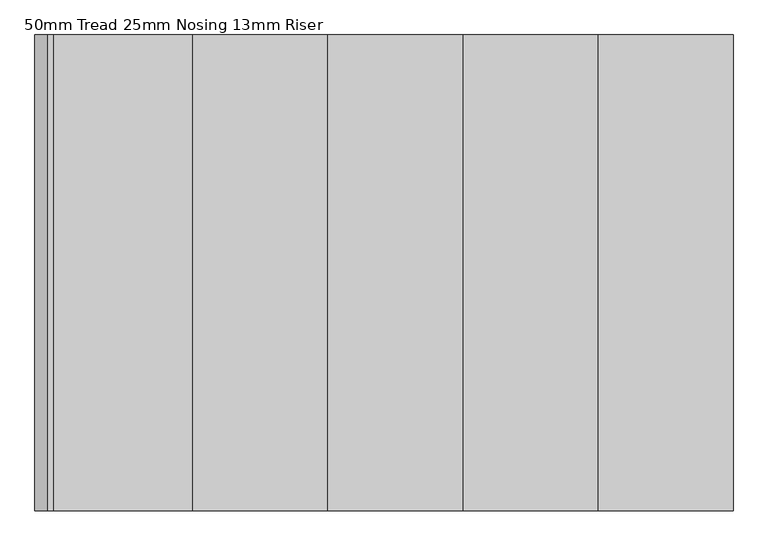
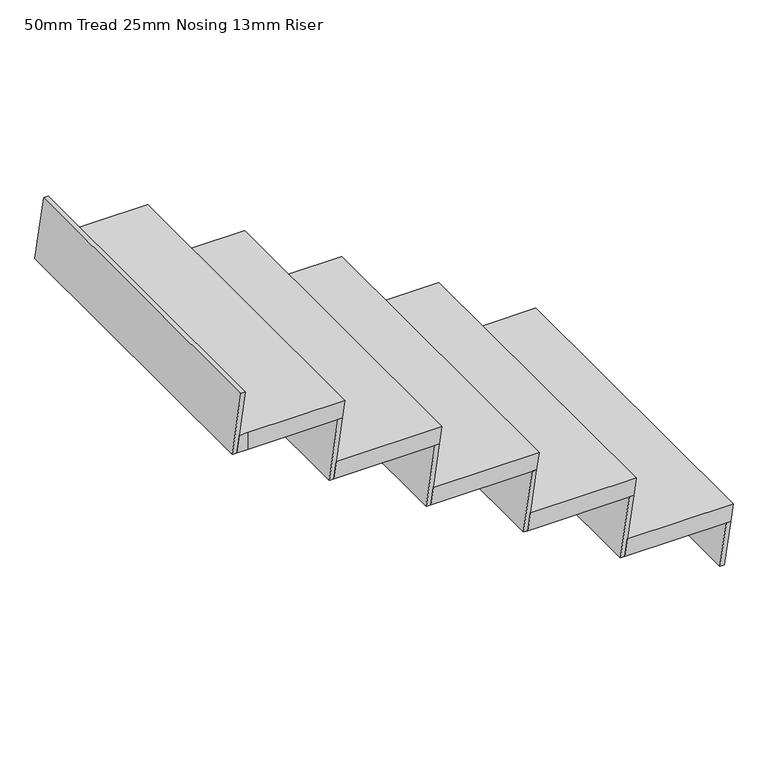
"""IFC4 building model written with IfcOpenShell, lengths in millimetres: stair flight geometry, 50mm Tread 25mm Nosing 13mm Riser."""

from ifc_helpers import new_model, si_unit, origin, place, context, project, spatial, faceted_brep, source, transform, mapped, element, save


def stair_flight_50mm_tread_25mm_nosing_13mm_riser_d346f2b6(model_context):
    return source(origin(), model_context, "Body", "Brep", [
        faceted_brep([(-839.0915237, 1810.8567276, 173.9130435), (-846.2790237, 1810.8567276, 123.9130435), (-846.2790237, 843.0180557, 123.9130435), (-839.0915237, 843.0180557, 173.9130435), (-539.0915237, 843.0180557, 173.9130435), (-539.0915237, 1810.8567276, 173.9130435), (-546.2790237, 1810.8567276, 123.9130435), (-546.2790237, 843.0180557, 123.9130435)], [[[0, 1, 2, 3]], [[3, 4, 5, 0]], [[2, 1, 6, 7]], [[4, 3, 2, 7]], [[0, 5, 6, 1]], [[5, 4, 7, 6]]]),
        faceted_brep([(-546.2790237, 1810.8567276, 123.9130435), (-564.0915237, 1810.8567276, 0.0), (-576.7200137, 1810.8567276, 0.0), (-558.9075137, 1810.8567276, 123.9130435), (-546.2790237, 843.0180557, 123.9130435), (-558.9075137, 843.0180557, 123.9130435), (-576.7200137, 843.0180557, 0.0), (-564.0915237, 843.0180557, 0.0)], [[[0, 1, 2, 3]], [[4, 5, 6, 7]], [[1, 0, 4, 7]], [[2, 1, 7, 6]], [[3, 2, 6, 5]], [[0, 3, 5, 4]]]),
        faceted_brep([(-821.2790237, 1810.8567276, 297.826087), (-846.2790237, 1810.8567276, 123.9130435), (-858.9075137, 1810.8567276, 123.9130435), (-833.9075137, 1810.8567276, 297.826087), (-821.2790237, 843.0180557, 297.826087), (-833.9075137, 843.0180557, 297.826087), (-858.9075137, 843.0180557, 123.9130435), (-846.2790237, 843.0180557, 123.9130435)], [[[0, 1, 2, 3]], [[4, 5, 6, 7]], [[1, 0, 4, 7]], [[2, 1, 7, 6]], [[3, 2, 6, 5]], [[0, 3, 5, 4]]]),
        faceted_brep([(-1114.0915237, 843.0180557, 347.826087), (-814.0915237, 843.0180557, 347.826087), (-814.0915237, 1810.8567276, 347.826087), (-1114.0915237, 1810.8567276, 347.826087), (-1121.2790237, 843.0180557, 297.826087), (-1121.2790237, 1810.8567276, 297.826087), (-821.2790237, 1810.8567276, 297.826087), (-821.2790237, 843.0180557, 297.826087)], [[[0, 1, 2, 3]], [[4, 5, 6, 7]], [[1, 0, 4, 7]], [[3, 2, 6, 5]], [[3, 5, 4, 0]], [[2, 1, 7, 6]]]),
        faceted_brep([(-1096.2790237, 1810.8567276, 471.7391304), (-1121.2790237, 1810.8567276, 297.826087), (-1133.9075137, 1810.8567276, 297.826087), (-1108.9075137, 1810.8567276, 471.7391304), (-1096.2790237, 843.0180557, 471.7391304), (-1108.9075137, 843.0180557, 471.7391304), (-1133.9075137, 843.0180557, 297.826087), (-1121.2790237, 843.0180557, 297.826087)], [[[0, 1, 2, 3]], [[4, 5, 6, 7]], [[1, 0, 4, 7]], [[2, 1, 7, 6]], [[3, 2, 6, 5]], [[0, 3, 5, 4]]]),
        faceted_brep([(-1389.0915237, 843.0180557, 521.7391304), (-1089.0915237, 843.0180557, 521.7391304), (-1089.0915237, 1810.8567276, 521.7391304), (-1389.0915237, 1810.8567276, 521.7391304), (-1396.2790237, 843.0180557, 471.7391304), (-1396.2790237, 1810.8567276, 471.7391304), (-1096.2790237, 1810.8567276, 471.7391304), (-1096.2790237, 843.0180557, 471.7391304)], [[[0, 1, 2, 3]], [[4, 5, 6, 7]], [[1, 0, 4, 7]], [[3, 2, 6, 5]], [[3, 5, 4, 0]], [[2, 1, 7, 6]]]),
        faceted_brep([(-1371.2790237, 1810.8567276, 645.6521739), (-1396.2790237, 1810.8567276, 471.7391304), (-1408.9075137, 1810.8567276, 471.7391304), (-1383.9075137, 1810.8567276, 645.6521739), (-1371.2790237, 843.0180557, 645.6521739), (-1383.9075137, 843.0180557, 645.6521739), (-1408.9075137, 843.0180557, 471.7391304), (-1396.2790237, 843.0180557, 471.7391304)], [[[0, 1, 2, 3]], [[4, 5, 6, 7]], [[1, 0, 4, 7]], [[2, 1, 7, 6]], [[3, 2, 6, 5]], [[0, 3, 5, 4]]]),
        faceted_brep([(-1664.0915237, 843.0180557, 695.6521739), (-1364.0915237, 843.0180557, 695.6521739), (-1364.0915237, 1810.8567276, 695.6521739), (-1664.0915237, 1810.8567276, 695.6521739), (-1671.2790237, 843.0180557, 645.6521739), (-1671.2790237, 1810.8567276, 645.6521739), (-1371.2790237, 1810.8567276, 645.6521739), (-1371.2790237, 843.0180557, 645.6521739)], [[[0, 1, 2, 3]], [[4, 5, 6, 7]], [[1, 0, 4, 7]], [[3, 2, 6, 5]], [[3, 5, 4, 0]], [[2, 1, 7, 6]]]),
        faceted_brep([(-1921.2790237, 1810.8567276, 993.4782609), (-1946.2790237, 1810.8567276, 819.5652174), (-1958.9075137, 1810.8567276, 819.5652174), (-1933.9075137, 1810.8567276, 993.4782609), (-1921.2790237, 843.0180557, 993.4782609), (-1933.9075137, 843.0180557, 993.4782609), (-1958.9075137, 843.0180557, 819.5652174), (-1946.2790237, 843.0180557, 819.5652174)], [[[0, 1, 2, 3]], [[4, 5, 6, 7]], [[1, 0, 4, 7]], [[2, 1, 7, 6]], [[3, 2, 6, 5]], [[0, 3, 5, 4]]]),
        faceted_brep([(-1646.2790237, 1810.8567276, 819.5652174), (-1671.2790237, 1810.8567276, 645.6521739), (-1683.9075137, 1810.8567276, 645.6521739), (-1658.9075137, 1810.8567276, 819.5652174), (-1646.2790237, 843.0180557, 819.5652174), (-1658.9075137, 843.0180557, 819.5652174), (-1683.9075137, 843.0180557, 645.6521739), (-1671.2790237, 843.0180557, 645.6521739)], [[[0, 1, 2, 3]], [[4, 5, 6, 7]], [[1, 0, 4, 7]], [[2, 1, 7, 6]], [[3, 2, 6, 5]], [[0, 3, 5, 4]]]),
        faceted_brep([(-1939.0915237, 843.0180557, 869.5652174), (-1914.0915237, 843.0180557, 869.5652174), (-1639.0915237, 843.0180557, 869.5652174), (-1639.0915237, 1810.8567276, 869.5652174), (-1939.0915237, 1810.8567276, 869.5652174), (-1946.2790237, 843.0180557, 819.5652174), (-1946.2790237, 1810.8567276, 819.5652174), (-1646.2790237, 1810.8567276, 819.5652174), (-1646.2790237, 843.0180557, 819.5652174), (-1914.0915237, 843.0180557, 819.5652174)], [[[0, 1, 2, 3, 4]], [[5, 6, 7, 8, 9]], [[1, 0, 5, 9]], [[2, 1, 9, 8]], [[4, 3, 7, 6]], [[4, 6, 5, 0]], [[3, 2, 8, 7]]]),
    ])


if __name__ == "__main__":
    model = new_model("IFC4")
    model_context = context("Model", 3, world=origin())
    ifc_project = project(units=[si_unit("LENGTHUNIT", "METRE", prefix="MILLI")], contexts=[model_context])
    site = spatial("IfcSite", under=ifc_project)
    building = spatial("IfcBuilding", under=site)
    placement = place(None, origin())
    stair_flight_50mm_tread_25mm_nosing_13mm_riser_shape = stair_flight_50mm_tread_25mm_nosing_13mm_riser_d346f2b6(model_context)
    element("IfcStairFlight", 1, ObjectType="50mm Tread 25mm Nosing 13mm Riser", at=placement, inside=building, context=model_context, shape_type="MappedRepresentation", body=[
        mapped(stair_flight_50mm_tread_25mm_nosing_13mm_riser_shape, transform((0.0, 0.0, 0.0), x_axis=(1.0, 0.0, 0.0), y_axis=(0.0, 1.0, 0.0), z_axis=(0.0, 0.0, 1.0))),
    ])
    save(model, "model.ifc")
